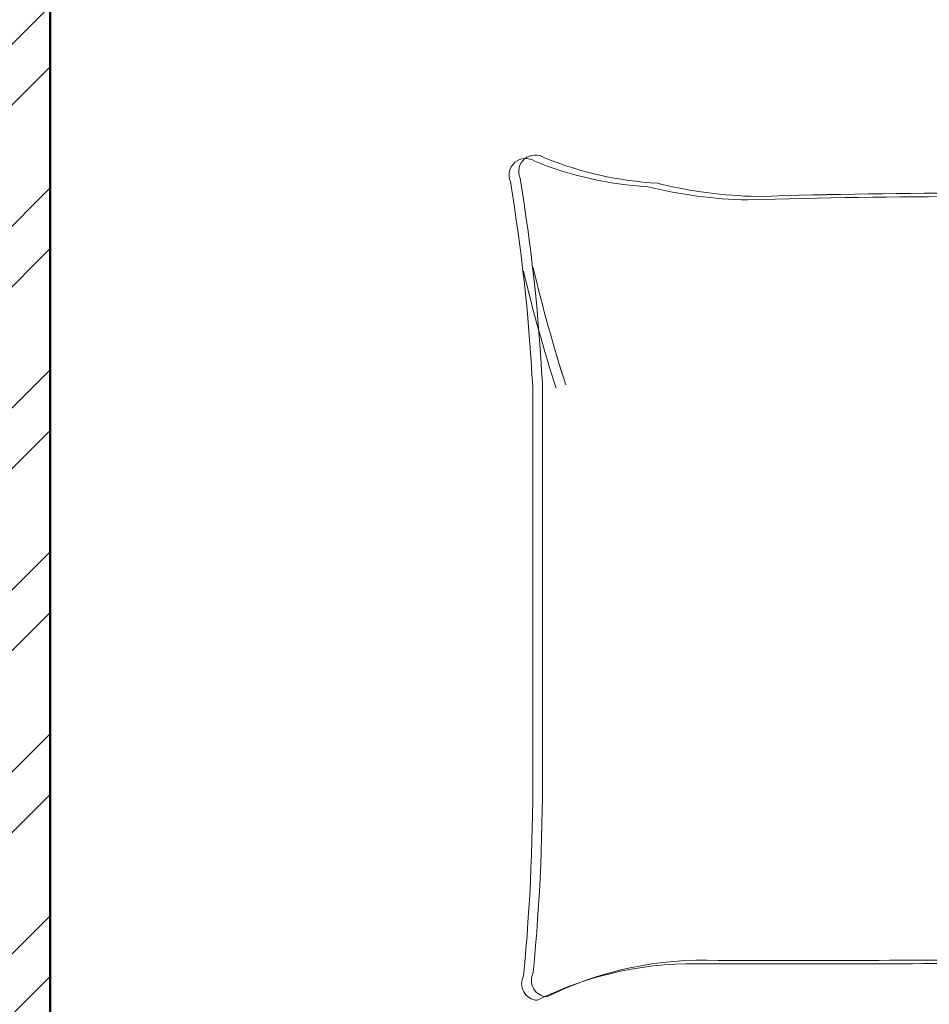
# Model space of a CAD drawing. Units: inches. Extents: x 1901 to 2863, y 888 to 2433.
# Tile 41 of 91: x 2618 to 2686, y 1563 to 1636. Entities that reach past the tile are written whole.
import ezdxf

# ---------------------------------------------------------------- set-up
doc = ezdxf.new("R2010")
doc.units = ezdxf.units.IN
for name, color, linetype, lineweight in [('A-FURN', 8, 'Continuous', 18), ('A-WALL', 7, 'Continuous', 50), ('A-WALL-PATT', 8, 'Continuous', 13)]:
    doc.layers.add(name, color=color, linetype=linetype, lineweight=lineweight)

# ---------------------------------------------------------------- blocks, each defined once
blk = doc.blocks.new('BED-DOUBLE')
for p, q in [((31.178, 59.321), (27.529, 55.161)), ((31.178, 59.32), (27.529, 55.16)), ((31.896, 59.577), (28.246, 55.417)), ((31.896, 59.577), (28.246, 55.417)), ((33.137, 59.41), (31.178, 59.321, 4.346)), ((33.137, 59.41), (31.178, 59.32, 4.346)), ((31.873, 57.595), (31.178, 59.321)), ((31.873, 57.595), (31.178, 59.32)), ((33.854, 59.666), (31.896, 59.577, 4.346)), ((33.854, 59.666), (31.896, 59.577, 4.346)), ((32.591, 57.851), (31.896, 59.577)), ((32.591, 57.851), (31.896, 59.577)), ((0.026, 57.778), (0.026, 4.122)), ((0.744, 57.778), (30.62, 57.778)), ((0.744, 57.778), (30.62, 57.778)), ((31.525, 54.117), (31.873, 57.595)), ((31.525, 54.117), (31.873, 57.595)), ((32.243, 54.374), (32.591, 57.851)), ((32.243, 54.373), (32.591, 57.851)), ((18.633, 56.885), (15.109, 56.014)), ((18.633, 56.885), (15.109, 56.014)), ((19.351, 57.142), (15.827, 56.271)), ((19.351, 57.141), (15.827, 56.271)), ((18.18, 51.123), (18.633, 56.885)), ((18.18, 51.123), (18.633, 56.885)), ((18.898, 51.38), (19.351, 57.142)), ((18.898, 51.379), (19.351, 57.141)), ((2.897, 56.227), (2.788, 50.161)), ((2.897, 56.227), (2.788, 50.161)), ((2.897, 56.227), (6.502, 55.801)), ((2.897, 56.227), (6.502, 55.802)), ((3.615, 56.483), (3.506, 50.417)), ((3.615, 56.483), (3.506, 50.418)), ((3.615, 56.483), (7.22, 56.058)), ((3.615, 56.483), (7.22, 56.058)), ((6.502, 55.801), (9.388, 56.47)), ((6.502, 55.802), (9.388, 56.47)), ((7.22, 56.058), (10.106, 56.726)), ((7.22, 56.058), (10.106, 56.726)), ((13.307, 56.227), (9.297, 55.326)), ((13.307, 56.227), (9.297, 55.326)), ((9.388, 56.47), (10.563, 55.893)), ((9.388, 56.47), (10.563, 55.893)), ((14.025, 56.483), (10.015, 55.582)), ((14.025, 56.483), (10.015, 55.582)), ((10.106, 56.726), (11.28, 56.149)), ((10.106, 56.726), (11.28, 56.149)), ((15.109, 56.014), (13.307, 56.227)), ((15.109, 56.014), (13.307, 56.227)), ((15.827, 56.271), (14.025, 56.483)), ((15.827, 56.271), (14.025, 56.483)), ((10.015, 55.582), (7.007, 54.256)), ((10.015, 55.582), (7.007, 54.256)), ((28.246, 55.417), (25.814, 52.113)), ((28.246, 55.417), (25.814, 52.113)), ((9.297, 55.326), (6.289, 53.999)), ((9.297, 55.326), (6.289, 54)), ((27.529, 55.161), (25.096, 51.857)), ((27.529, 55.16), (25.096, 51.856)), ((31.873, 49.77), (31.525, 54.117)), ((31.873, 49.77), (31.525, 54.117)), ((32.591, 50.027), (32.243, 54.374)), ((32.591, 50.026), (32.243, 54.373)), ((25.096, 51.857), (22.837, 45.597)), ((25.096, 51.856), (22.837, 45.597)), ((25.814, 52.113), (23.554, 45.853)), ((25.814, 52.113), (23.554, 45.853)), ((2.788, 50.161), (2.881, 51.287)), ((2.788, 50.161), (2.881, 51.287)), ((2.881, 51.287), (3.472, 47.023)), ((2.881, 51.287), (3.472, 47.023)), ((3.506, 50.418), (3.598, 51.544)), ((3.506, 50.417), (3.598, 51.543)), ((3.598, 51.544), (4.19, 47.279)), ((3.598, 51.543), (4.19, 47.279)), ((18.806, 48.922), (18.18, 51.123)), ((18.806, 48.922), (18.18, 51.123)), ((19.523, 49.179), (18.898, 51.38)), ((19.523, 49.179), (18.898, 51.379)), ((32.394, 45.945), (31.873, 49.77)), ((32.394, 45.944), (31.873, 49.77)), ((33.112, 46.201), (32.591, 50.027)), ((33.112, 46.201), (32.591, 50.026)), ((18.322, 41.052), (18.806, 48.922)), ((18.322, 41.052), (18.806, 48.922)), ((19.039, 41.308), (19.523, 49.179)), ((19.039, 41.308), (19.523, 49.179)), ((3.472, 47.023), (4.991, 40.938)), ((3.472, 47.023), (4.991, 40.938)), ((4.19, 47.279), (5.709, 41.195)), ((4.19, 47.279), (5.709, 41.195)), ((33.437, 43.684), (32.394, 45.945)), ((33.437, 43.684), (32.394, 45.944)), ((34.155, 43.941), (33.112, 46.201)), ((34.155, 43.94), (33.112, 46.201)), ((22.837, 45.597), (19.543, 36.235)), ((22.837, 45.597), (19.543, 36.235)), ((23.554, 45.853), (20.261, 36.492)), ((23.554, 45.853), (20.261, 36.491)), ((88.998, 16.876), (88.998, 44.511)), ((88.998, 16.876), (88.998, 44.511)), ((89.716, 17.132), (89.716, 44.768)), ((89.716, 17.132), (89.716, 44.767)), ((4.151, 43.976), (3.482, 41.657)), ((4.151, 43.975), (3.482, 41.657)), ((4.869, 44.232), (4.2, 41.913)), ((4.869, 44.232), (4.2, 41.914)), ((34.85, 41.158), (34.155, 43.941)), ((34.85, 41.158), (34.155, 43.94)), ((34.132, 40.902), (33.437, 43.684)), ((34.132, 40.902), (33.437, 43.684)), ((3.482, 41.657), (2.875, 38.367)), ((3.482, 41.657), (2.875, 38.367)), ((4.2, 41.914), (3.593, 38.623)), ((4.2, 41.913), (3.593, 38.623)), ((17.573, 36.525), (18.322, 41.052)), ((17.573, 36.525), (18.322, 41.052)), ((18.291, 36.782), (19.039, 41.308)), ((18.291, 36.781), (19.039, 41.308)), ((31.873, 40.554), (34.132, 40.902)), ((31.873, 40.554), (34.132, 40.902)), ((32.591, 40.811), (34.85, 41.158)), ((32.591, 40.81), (34.85, 41.158)), ((26.834, 38.642), (31.873, 40.554)), ((26.834, 38.641), (31.873, 40.554)), ((27.551, 38.898), (32.591, 40.811)), ((27.551, 38.898), (32.591, 40.81)), ((19.543, 33.937), (26.834, 38.642)), ((19.543, 33.937), (26.834, 38.641)), ((20.261, 34.194), (27.551, 38.898)), ((20.261, 34.193), (27.551, 38.898)), ((2.875, 38.367), (2.897, 38.006)), ((2.875, 38.367), (2.897, 38.007)), ((2.897, 38.007), (3.371, 33.035)), ((2.897, 38.006), (3.371, 33.035)), ((3.593, 38.623), (3.615, 38.263)), ((3.593, 38.623), (3.615, 38.263)), ((3.615, 38.263), (4.088, 33.291)), ((3.615, 38.263), (4.088, 33.291)), ((18.82, 34.489), (17.378, 37.936)), ((18.82, 34.488), (17.378, 37.936)), ((19.538, 34.745), (18.096, 38.192)), ((19.538, 34.745), (18.096, 38.192)), ((18.993, 31.735), (18.82, 34.489)), ((18.993, 31.734), (18.82, 34.488)), ((19.71, 31.991), (19.538, 34.745)), ((19.71, 31.991), (19.538, 34.745)), ((3.371, 33.035), (2.824, 31.374)), ((3.371, 33.035), (2.824, 31.375)), ((4.088, 33.291), (3.542, 31.631)), ((4.088, 33.291), (3.542, 31.631)), ((2.824, 31.375), (8.859, 31.101)), ((2.824, 31.374), (8.859, 31.101)), ((3.542, 31.631), (9.577, 31.358)), ((3.542, 31.631), (9.577, 31.358)), ((9.577, 31.358), (13.182, 30.933)), ((9.577, 31.358), (13.182, 30.932)), ((13.922, 30.767), (15.988, 31.547)), ((13.922, 30.767), (15.988, 31.547)), ((14.64, 31.024), (16.706, 31.803)), ((14.64, 31.024), (16.706, 31.803)), ((15.988, 31.547), (18.993, 31.735)), ((15.988, 31.547), (18.993, 31.734)), ((16.706, 31.803), (19.71, 31.991)), ((16.706, 31.803), (19.71, 31.991)), ((8.85, 30.041), (12.422, 30.69)), ((8.85, 30.041), (12.422, 30.69)), ((8.859, 31.101), (12.464, 30.676)), ((8.859, 31.101), (12.464, 30.676)), ((12.422, 30.69), (13.883, 30.69)), ((12.422, 30.69), (13.883, 30.69)), ((12.464, 30.676), (13.922, 30.767)), ((12.464, 30.676), (13.922, 30.767)), ((13.182, 30.932), (14.64, 31.024)), ((13.182, 30.933), (14.64, 31.024)), ((13.883, 30.69), (15.993, 30.041)), ((13.883, 30.69), (15.993, 30.041)), ((2.844, 29.392), (8.85, 30.041)), ((2.844, 29.392), (8.85, 30.041)), ((8.132, 29.785), (11.704, 30.434)), ((8.132, 29.784), (11.704, 30.434)), ((11.704, 30.434), (13.165, 30.434)), ((11.704, 30.434), (13.165, 30.434)), ((13.165, 30.434), (15.275, 29.785)), ((13.165, 30.434), (15.275, 29.784)), ((15.993, 30.041), (19.003, 30.041)), ((15.993, 30.041), (19.003, 30.041)), ((19.003, 30.041), (19.003, 27.282)), ((19.003, 30.041), (19.003, 27.282)), ((2.126, 29.136), (8.132, 29.785)), ((2.126, 29.135), (8.132, 29.784)), ((3.493, 27.769), (2.844, 29.392)), ((3.493, 27.769), (2.844, 29.392)), ((15.275, 29.785), (18.286, 29.785)), ((15.275, 29.784), (18.286, 29.784)), ((18.286, 29.785), (18.286, 27.026)), ((18.286, 29.784), (18.286, 27.025)), ((2.775, 27.513), (2.126, 29.136)), ((2.775, 27.512), (2.126, 29.135)), ((3.331, 22.777), (3.493, 27.769)), ((3.331, 22.778), (3.493, 27.769)), ((18.898, 21.983), (19.351, 27.745)), ((18.898, 21.983), (19.351, 27.745)), ((2.613, 22.521), (2.775, 27.513)), ((2.613, 22.521), (2.775, 27.512)), ((18.286, 27.026), (17.061, 23.495)), ((18.286, 27.025), (17.061, 23.495)), ((19.003, 27.282), (17.779, 23.752)), ((19.003, 27.282), (17.779, 23.751)), ((18.18, 21.727), (18.633, 27.489)), ((18.18, 21.727), (18.633, 27.488)), ((3.331, 22.417), (3.331, 22.778)), ((3.331, 22.416), (3.331, 22.777)), ((2.613, 22.16), (2.613, 22.521)), ((2.613, 22.16), (2.613, 22.521)), ((3.425, 18.914), (2.613, 22.16)), ((3.425, 18.914), (2.613, 22.16)), ((4.142, 19.171), (3.331, 22.417)), ((4.142, 19.17), (3.331, 22.416)), ((19.523, 19.782), (18.898, 21.983)), ((19.523, 19.782), (18.898, 21.983)), ((18.806, 19.526), (18.18, 21.727)), ((18.806, 19.526), (18.18, 21.727)), ((3.749, 13.558), (4.886, 19.726)), ((3.749, 13.558), (4.886, 19.725)), ((4.467, 13.815), (5.603, 19.982)), ((4.467, 13.814), (5.603, 19.982)), ((19.039, 11.912), (19.523, 19.782)), ((19.039, 11.912), (19.523, 19.782)), ((4.954, 16.898), (4.142, 19.171)), ((4.954, 16.898), (4.142, 19.17)), ((18.322, 11.656), (18.806, 19.526)), ((18.322, 11.655), (18.806, 19.526)), ((4.236, 16.642), (3.425, 18.914)), ((4.236, 16.642), (3.425, 18.914)), ((3.425, 9.265), (3.749, 13.558)), ((3.425, 9.265), (3.749, 13.558)), ((4.142, 9.522), (4.467, 13.815)), ((4.142, 9.522), (4.467, 13.814)), ((18.291, 7.385), (19.039, 11.912)), ((18.291, 7.385), (19.039, 11.912)), ((19.039, 11.912), (19.402, 10.639)), ((19.039, 11.912), (19.402, 10.64)), ((17.573, 7.129), (18.322, 11.656)), ((17.573, 7.128), (18.322, 11.655)), ((18.322, 11.656), (18.684, 10.383)), ((18.322, 11.655), (18.684, 10.383)), ((18.684, 10.383), (19.496, 4.661)), ((18.684, 10.383), (19.496, 4.661)), ((19.402, 10.64), (20.214, 4.917)), ((19.402, 10.639), (20.214, 4.917)), ((4.122, 9.403), (4.142, 9.522)), ((4.122, 9.404), (4.142, 9.522)), ((3.404, 9.147), (3.425, 9.265)), ((3.404, 9.147), (3.425, 9.265)), ((3.774, 4.341), (3.404, 9.147)), ((3.774, 4.341), (3.404, 9.147)), ((4.492, 4.597), (4.122, 9.404)), ((4.492, 4.597), (4.122, 9.403)), ((10.08, 5.635), (6.996, 6.771)), ((10.08, 5.634), (6.996, 6.771)), ((10.798, 5.891), (7.714, 7.027)), ((10.798, 5.891), (7.714, 7.027)), ((14.857, 5.242), (10.798, 5.891)), ((14.857, 5.242), (10.798, 5.891)), ((4.467, 4.592), (8.039, 5.242)), ((4.467, 4.593), (8.038, 5.242)), ((8.038, 5.242), (10.961, 4.755)), ((8.039, 5.242), (10.961, 4.755)), ((14.139, 4.986), (10.08, 5.635)), ((14.139, 4.985), (10.08, 5.634)), ((10.243, 4.498), (11.379, 5.148)), ((10.243, 4.499), (11.379, 5.148)), ((10.961, 4.755), (12.097, 5.404)), ((10.961, 4.755), (12.097, 5.404)), ((15.925, 5.31), (14.139, 4.985)), ((15.924, 5.31), (14.139, 4.986)), ((16.642, 5.567), (14.857, 5.242)), ((16.642, 5.566), (14.857, 5.242)), ((19.496, 4.661), (15.924, 5.31)), ((19.496, 4.661), (15.925, 5.31)), ((20.214, 4.917), (16.642, 5.567)), ((20.214, 4.917), (16.642, 5.566)), ((3.749, 4.336), (7.321, 4.986)), ((3.749, 4.336), (7.321, 4.985)), ((7.321, 4.986), (10.243, 4.499)), ((7.321, 4.985), (10.243, 4.498))]:
    blk.add_line(p, q)
for centre, radius, start, end in [((77.121, 85.469), 25.896, 267.47137, 296.46809), ((77.121, 85.469), 25.896, 267.47137, 296.46809), ((77.839, 85.726), 25.896, 267.47137, 296.46809), ((77.839, 85.725), 25.896, 267.47137, 296.46809), ((88.578, 61.052), 1.238, 332.65876, 86.02002), ((88.578, 61.052), 1.238, 332.65876, 86.02002), ((89.295, 61.309), 1.238, 332.65876, 86.02002), ((89.295, 61.308), 1.238, 332.65876, 86.02002), ((239.077, 46.423), 149.37, 174.4998, 180.63509), ((239.077, 46.423), 149.37, 174.4998, 180.63509), ((41.517, 204.859), 145.395, 266.97912, 273.83645), ((41.517, 204.859), 145.395, 266.97912, 273.83645), ((76.89, -5061.969), 5121.824, 90.002168, 90.286888), ((76.89, -5061.97), 5121.824, 90.002168, 90.286888), ((238.36, 46.167), 149.37, 174.4998, 180.63509), ((238.36, 46.167), 149.37, 174.4998, 180.63509), ((-7.447, 57.591), 40.624, 349.87628, 2.56571), ((-7.447, 57.591), 40.624, 349.87628, 2.56571), ((40.799, 204.603), 145.395, 266.97912, 273.83645), ((40.799, 204.602), 145.395, 266.97912, 273.83645), ((-6.729, 57.848), 40.624, 349.87628, 2.56571), ((-6.729, 57.847), 40.624, 349.87628, 2.56571), ((76.173, -5062.226), 5121.824, 90.002168, 90.286888), ((76.173, -5062.226), 5121.824, 90.002168, 90.286888), ((39.397, 49.077), 6.988, 168.6608, 203.73842), ((39.397, 49.076), 6.988, 168.6608, 203.73842), ((40.115, 49.333), 6.988, 168.6608, 203.73842), ((40.115, 49.333), 6.988, 168.6608, 203.73842), ((1.69, 34.942), 33.294, 10.66171, 19.88058), ((1.69, 34.941), 33.294, 10.66171, 19.88058), ((2.408, 35.198), 33.294, 10.66171, 19.88058), ((2.408, 35.198), 33.294, 10.66171, 19.88058), ((176.248, 20.155), 144.857, 171.78449, 186.90062), ((176.248, 20.155), 144.857, 171.78449, 186.90062), ((34.202, 41.097), 0.207, 250.24637, 1.13765), ((34.202, 41.097), 0.207, 250.24637, 1.13765), ((34.92, 41.353), 0.207, 250.24637, 1.13765), ((34.92, 41.353), 0.207, 250.24637, 1.13765), ((175.53, 19.899), 144.857, 171.78449, 186.90062), ((175.53, 19.899), 144.857, 171.78449, 186.90062), ((204.426, 23.944), 185.219, 176.08655, 186.78213), ((204.426, 23.944), 185.219, 176.08655, 186.78213), ((205.143, 24.201), 185.219, 176.08655, 186.78213), ((205.143, 24.2), 185.219, 176.08655, 186.78213), ((225.516, 24.021), 136.704, 182.99578, 189.40907), ((225.516, 24.02), 136.704, 182.99578, 189.40907), ((226.234, 24.277), 136.704, 182.99578, 189.40907), ((226.234, 24.277), 136.704, 182.99578, 189.40907), ((35.026, -187.881), 190.991, 88.4762, 91.00819), ((35.026, -187.881), 190.991, 88.4762, 91.00819), ((35.744, -187.624), 190.991, 88.4762, 91.00819), ((35.744, -187.625), 190.991, 88.4762, 91.00819), ((56.853, 544.298), 541.514, 268.22771, 271.71854), ((56.853, 544.297), 541.514, 268.22771, 271.71854), ((57.571, 544.554), 541.514, 268.22771, 271.71854), ((57.571, 544.554), 541.514, 268.22771, 271.71854), ((72.461, -30.238), 33.271, 76.06484, 88.91125), ((72.461, -30.238), 33.271, 76.06484, 88.91125), ((73.178, -29.981), 33.271, 76.06484, 88.91125), ((73.178, -29.982), 33.271, 76.06484, 88.91125), ((22.589, 95.579), 93.531, 268.72178, 275.60397), ((22.589, 95.579), 93.531, 268.72178, 275.60397), ((23.307, 95.835), 93.531, 268.72178, 275.60397), ((23.307, 95.835), 93.531, 268.72178, 275.60397), ((79.646, -24.098), 26.454, 67.97508, 86.652), ((79.646, -24.098), 26.454, 67.97508, 86.652), ((78.928, -24.355), 26.454, 67.97508, 86.652), ((78.928, -24.355), 26.454, 67.97508, 86.652), ((89.529, 1.185), 1.223, 236.17358, 23.47814), ((89.529, 1.184), 1.223, 236.17358, 23.47814), ((90.247, 1.441), 1.223, 236.17358, 23.47814), ((90.247, 1.441), 1.223, 236.17358, 23.47814)]:
    blk.add_arc(centre, radius, start, end)

msp = doc.modelspace()

# ---------------------------------------------------------------- hatches: boundary and pattern name
at = {"layer": 'A-WALL-PATT'}
h = msp.add_hatch(dxfattribs=at)
h.set_pattern_fill('ANSI32', color=256)
h.paths.add_polyline_path([(2443.926, 2139.888), (2439.426, 2139.888), (2439.426, 2069.348), (2441.676, 2069.348), (2443.926, 2069.348), (2443.926, 2078.634), (2521.926, 2078.634), (2521.926, 2075.067), (2524.176, 2075.067), (2526.426, 2075.067), (2526.426, 2078.634), (2571.755, 2078.634), (2571.755, 2080.884), (2571.755, 2083.134), (2443.926, 2083.134)])
h.paths.add_polyline_path([(2526.426, 2054.634), (2524.176, 2054.634), (2521.926, 2054.634), (2521.926, 2030.634), (2443.926, 2030.634), (2443.926, 2045.348), (2439.426, 2045.348), (2439.426, 1983.867), (2443.926, 1983.867), (2443.926, 2026.134), (2521.926, 2026.134), (2526.426, 2026.134)])
h.paths.add_polyline_path([(2443.926, 1923.867), (2439.426, 1923.867), (2439.426, 1872.634), (2443.926, 1872.634)])
h.paths.add_polyline_path([(2636.233, 1766.134), (2609.926, 1766.134), (2609.926, 1779.785), (2605.426, 1779.785), (2605.426, 1766.134), (2486.614, 1766.134), (2486.614, 1770.671), (2482.114, 1770.671), (2482.114, 1766.134), (2482.114, 1761.634), (2636.233, 1761.634), (2636.233, 1763.884)])
h.paths.add_polyline_path([(2519.536, 1663.384), (2519.536, 1665.634), (2494.926, 1665.634), (2481.831, 1665.634), (2481.831, 1663.384), (2481.831, 1661.134), (2490.426, 1661.134), (2490.426, 1640.157), (2494.926, 1640.157), (2494.926, 1661.134), (2519.536, 1661.134)])
h.paths.add_polyline_path([(2443.926, 1712.134), (2443.926, 1716.634), (2414.464, 1716.634), (2414.464, 1712.134), (2439.426, 1712.134), (2439.426, 1545.507), (2443.926, 1545.507), (2443.926, 1661.134), (2448.475, 1661.134), (2448.475, 1665.634), (2443.926, 1665.634)])
h.paths.add_polyline_path([(2343.426, 1712.134), (2365.525, 1712.134), (2365.525, 1714.384), (2365.525, 1716.634), (2333.871, 1716.634), (2333.871, 1714.384), (2333.871, 1712.134), (2338.926, 1712.134), (2338.926, 1575.634), (2338.926, 1545.507), (2343.426, 1545.507), (2343.426, 1547.507), (2343.426, 1580.134)])
h.paths.add_polyline_path([(2752.926, 1665.634), (2579.536, 1665.634), (2579.536, 1661.134), (2615.926, 1661.134), (2615.926, 1529.134), (2598.931, 1529.134), (2598.931, 1524.634), (2623.127, 1524.634), (2623.127, 1526.884), (2623.127, 1529.134), (2620.426, 1529.134), (2620.426, 1661.134), (2748.426, 1661.134), (2748.426, 1633.499), (2752.926, 1633.499)])
h.paths.add_polyline_path([(2752.926, 1419.929), (2748.426, 1419.929), (2748.426, 1400.134), (2659.426, 1400.134), (2659.426, 1444.333), (2657.176, 1444.333), (2654.926, 1444.333), (2654.926, 1400.134), (2643.649, 1400.134), (2643.649, 1395.634), (2748.426, 1395.634), (2748.426, 1364.035), (2752.926, 1364.035)])
h.paths.add_polyline_path([(2752.926, 1492.878), (2748.426, 1492.878), (2748.426, 1476.634), (2667.426, 1476.634), (2667.426, 1479.71), (2665.176, 1479.71), (2662.926, 1479.71), (2662.926, 1476.634), (2654.926, 1476.634), (2654.926, 1469.536), (2659.426, 1469.536), (2659.426, 1472.134), (2748.426, 1472.134), (2748.426, 1455.929), (2752.926, 1455.929)])
h.paths.add_polyline_path([(2752.926, 1304.035), (2748.426, 1304.035), (2748.426, 1263.634), (2738.66, 1263.634), (2738.66, 1259.134), (2752.926, 1259.134)])
h.paths.add_polyline_path([(2685.926, 1259.134), (2695.49, 1259.134), (2695.49, 1261.384), (2695.49, 1263.634), (2677.837, 1263.634), (2677.837, 1261.384), (2677.837, 1259.134), (2681.426, 1259.134), (2681.426, 1203.634), (2653.277, 1203.634), (2653.277, 1199.134), (2685.926, 1199.134), (2685.926, 1203.634)])
h.paths.add_polyline_path([(2609.426, 1395.634), (2611.848, 1395.634), (2611.848, 1400.134), (2598.888, 1400.134), (2598.888, 1397.884), (2598.888, 1395.634), (2604.926, 1395.634), (2604.926, 1268.134), (2554.726, 1268.134), (2554.726, 1265.884), (2554.726, 1263.634), (2604.926, 1263.634), (2604.926, 1203.634), (2571.306, 1203.634), (2571.306, 1199.134), (2604.926, 1199.134), (2629.277, 1199.134), (2629.277, 1201.384), (2629.277, 1203.634), (2609.426, 1203.634), (2609.426, 1258.634), (2609.426, 1259.134), (2654.804, 1259.134), (2654.804, 1263.634), (2609.426, 1263.634)])
h.paths.add_polyline_path([(2443.926, 1304.035), (2439.426, 1304.035), (2439.426, 1259.134), (2443.926, 1259.134), (2456.16, 1259.134), (2456.16, 1261.384), (2456.16, 1263.634), (2443.926, 1263.634)])
h.paths.add_polyline_path([(2525.426, 1263.634), (2531.778, 1263.634), (2531.778, 1268.134), (2520.926, 1268.134), (2520.926, 1263.634), (2511.409, 1263.634), (2511.409, 1259.134), (2520.926, 1259.134), (2520.926, 1199.134), (2547.306, 1199.134), (2547.306, 1201.384), (2547.306, 1203.634), (2525.426, 1203.634)])
h.paths.add_polyline_path([(2443.926, 1434.842), (2439.426, 1434.842), (2439.426, 1364.035), (2441.676, 1364.035), (2443.926, 1364.035)])
h.paths.add_polyline_path([(2567.134, 1400.134), (2443.926, 1400.134), (2443.926, 1395.634), (2567.134, 1395.634)])
h.paths.add_polyline_path([(2443.926, 1545.507), (2439.426, 1545.507), (2439.426, 1494.842), (2443.926, 1494.842)])
h.paths.add_polyline_path([(2494.926, 1553.349), (2492.676, 1553.349), (2490.426, 1553.349), (2490.426, 1524.634), (2494.926, 1524.634), (2525.936, 1524.634), (2525.936, 1526.884), (2525.936, 1529.134), (2494.926, 1529.134)])
h.paths.add_polyline_path([(2752.926, 1573.499), (2748.426, 1573.499), (2748.426, 1529.134), (2657.759, 1529.134), (2657.759, 1524.634), (2662.926, 1524.634), (2662.926, 1498.631), (2667.426, 1498.631), (2667.426, 1524.634), (2748.426, 1524.634), (2748.426, 1516.878), (2752.926, 1516.878)])
h.paths.add_polyline_path([(2038.602, 2237.418), (2080.174, 2237.418), (2080.174, 2256.075), (2038.602, 2256.075)], flags=9)
h.paths.add_polyline_path([(2292.009, 1062.394), (2539.932, 1062.394), (2539.932, 1099.487), (2292.009, 1099.487)], flags=9)
h.paths.add_polyline_path([(2424.91, 1832.253), (2448.513, 1832.253), (2448.513, 1846.678), (2424.91, 1846.678)], flags=9)
h.paths.add_polyline_path([(2359.076, 1832.253), (2382.678, 1832.253), (2382.678, 1846.678), (2359.076, 1846.678)], flags=9)
h.paths.add_polyline_path([(2352.899, 1684.802), (2367.543, 1684.802), (2367.543, 1697.167), (2352.899, 1697.167)], flags=9)
h.paths.add_polyline_path([(2079.288, 1755.826), (2169.024, 1755.826), (2169.024, 1774.372), (2079.288, 1774.372)], flags=9)
h.paths.add_polyline_path([(2404.09, 1373.857), (2404.09, 1463.593), (2385.544, 1463.593), (2385.544, 1373.857)], flags=9)
h.paths.add_polyline_path([(2268.091, 2236.371), (2309.636, 2236.371), (2309.636, 2255.028), (2268.091, 2255.028)], flags=9)
h.paths.add_polyline_path([(2575.96, 1700.951), (2665.696, 1700.951), (2665.696, 1719.498), (2575.96, 1719.498)], flags=9)
h.paths.add_polyline_path([(2302.962, 1878.474), (2329.524, 1878.474), (2329.524, 1888.777), (2302.962, 1888.777)], flags=9)
h.paths.add_polyline_path([(2097.415, 2240.576), (2126.573, 2240.576), (2126.573, 2259.233), (2097.415, 2259.233)], flags=9)
h.paths.add_polyline_path([(2208.725, 2246.124), (2237.882, 2246.124), (2237.882, 2264.781), (2208.725, 2264.781)], flags=9)
h.paths.add_polyline_path([(2038.147, 1925.958), (2076.987, 1925.958), (2076.987, 1944.615), (2038.147, 1944.615)], flags=9)
h.paths.add_polyline_path([(2239.144, 1926.672), (2288.465, 1926.672), (2288.465, 1945.329), (2239.144, 1945.329)], flags=9)
h.paths.add_polyline_path([(2175.429, 2007.33), (2212.356, 2007.33), (2212.356, 2025.987), (2175.429, 2025.987)], flags=9)
h.paths.add_polyline_path([(2225.034, 2091.794), (2263.875, 2091.794), (2263.875, 2110.451), (2225.034, 2110.451)], flags=9)
h.paths.add_polyline_path([(2035.398, 2098.478), (2074.238, 2098.478), (2074.238, 2117.135), (2035.398, 2117.135)], flags=9)
h.paths.add_polyline_path([(2050.102, 2029.209), (2083.26, 2029.209), (2083.26, 2047.866), (2050.102, 2047.866)], flags=9)
h.paths.add_polyline_path([(2069.677, 1956.719), (2098.835, 1956.719), (2098.835, 1975.376), (2069.677, 1975.376)], flags=9)
h.paths.add_polyline_path([(2328.62, 1753.336), (2361.663, 1753.336), (2361.663, 1771.993), (2328.62, 1771.993)], flags=9)
h.paths.add_polyline_path([(2395.162, 2060.888), (2395.162, 2140.654), (2378.676, 2140.654), (2378.676, 2060.888)], flags=9)
h.paths.add_polyline_path([(2463.728, 2059.02), (2492.886, 2059.02), (2492.886, 2077.677), (2463.728, 2077.677)], flags=9)
h.paths.add_polyline_path([(2458.027, 2181.536), (2496.868, 2181.536), (2496.868, 2200.194), (2458.027, 2200.194)], flags=9)
h.paths.add_polyline_path([(2456.855, 2228.831), (2498.401, 2228.831), (2498.401, 2247.488), (2456.855, 2247.488)], flags=9)
h.paths.add_polyline_path([(2527.577, 2243.074), (2556.735, 2243.074), (2556.735, 2261.731), (2527.577, 2261.731)], flags=9)
h.paths.add_polyline_path([(2694.461, 2232.767), (2736.033, 2232.767), (2736.033, 2251.425), (2694.461, 2251.425)], flags=9)
h.paths.add_polyline_path([(2637.821, 2249.225), (2666.979, 2249.225), (2666.979, 2267.882), (2637.821, 2267.882)], flags=9)
h.paths.add_polyline_path([(2623.687, 2183.541), (2662.528, 2183.541), (2662.528, 2202.199), (2623.687, 2202.199)], flags=9)
h.paths.add_polyline_path([(2691.965, 2021.5), (2725.124, 2021.5), (2725.124, 2040.157), (2691.965, 2040.157)], flags=9)
h.paths.add_polyline_path([(2621.043, 1975.912), (2662.335, 1975.912), (2662.335, 1994.569), (2621.043, 1994.569)], flags=9)
h.paths.add_polyline_path([(2479.032, 1927.62), (2519.844, 1927.62), (2519.844, 1946.277), (2479.032, 1946.277)], flags=9)
h.paths.add_polyline_path([(2670.941, 1849.076), (2716.005, 1849.076), (2716.005, 1867.734), (2670.941, 1867.734)], flags=9)
h.paths.add_polyline_path([(2523.613, 1782.956), (2550.175, 1782.956), (2550.175, 1793.26), (2523.613, 1793.26)], flags=9)
h.paths.add_polyline_path([(2450.841, 1207.331), (2492.386, 1207.331), (2492.386, 1225.989), (2450.841, 1225.989)], flags=9)
h.paths.add_polyline_path([(2527.751, 1203.841), (2556.908, 1203.841), (2556.908, 1222.499), (2527.751, 1222.499)], flags=9)
h.paths.add_polyline_path([(2639.111, 1207.2), (2668.268, 1207.2), (2668.268, 1225.857), (2639.111, 1225.857)], flags=9)
h.paths.add_polyline_path([(2692.594, 1218.965), (2734.167, 1218.965), (2734.167, 1237.623), (2692.594, 1237.623)], flags=9)
h.paths.add_polyline_path([(2669.266, 1366.329), (2708.106, 1366.329), (2708.106, 1384.987), (2669.266, 1384.987)], flags=25)
h.paths.add_polyline_path([(2463.313, 1358.031), (2502.153, 1358.031), (2502.153, 1376.688), (2463.313, 1376.688)], flags=9)
h.paths.add_polyline_path([(2494.725, 1449.963), (2531.652, 1449.963), (2531.652, 1468.62), (2494.725, 1468.62)], flags=9)
h.paths.add_polyline_path([(2675.565, 1422.157), (2708.724, 1422.157), (2708.724, 1440.815), (2675.565, 1440.815)], flags=25)
h.paths.add_polyline_path([(2685.634, 1493.891), (2714.792, 1493.891), (2714.792, 1512.548), (2685.634, 1512.548)], flags=9)
h.paths.add_polyline_path([(2686.805, 1529.913), (2725.645, 1529.913), (2725.645, 1548.57), (2686.805, 1548.57)], flags=25)
h.paths.add_polyline_path([(2503.651, 1537.991), (2552.972, 1537.991), (2552.972, 1556.648), (2503.651, 1556.648)], flags=9)
h.paths.add_polyline_path([(2291.713, 1643.504), (2318.275, 1643.504), (2318.275, 1653.807), (2291.713, 1653.807)], flags=9)
h.paths.add_polyline_path([(2450.626, 1610.52), (2477.189, 1610.52), (2477.189, 1620.824), (2450.626, 1620.824)], flags=9)
h.paths.add_polyline_path([(2359.985, 1551.814), (2422.253, 1551.814), (2422.253, 1562.117), (2359.985, 1562.117)], flags=9)
h.paths.add_polyline_path([(2280.106, 1249.006), (2321.651, 1249.006), (2321.651, 1267.663), (2280.106, 1267.663)], flags=9)
h.paths.add_polyline_path([(2164.057, 1274.232), (2193.215, 1274.232), (2193.215, 1292.889), (2164.057, 1292.889)], flags=9)
h.paths.add_polyline_path([(2118.21, 1277.694), (2151.252, 1277.694), (2151.252, 1296.351), (2118.21, 1296.351)], flags=9)
h.paths.add_polyline_path([(2031.946, 1268.529), (2073.519, 1268.529), (2073.519, 1287.187), (2031.946, 1287.187)], flags=9)
h.paths.add_polyline_path([(2050.199, 1409.079), (2089.04, 1409.079), (2089.04, 1427.736), (2050.199, 1427.736)], flags=9)
h.paths.add_polyline_path([(2243.743, 1421.032), (2282.584, 1421.032), (2282.584, 1439.689), (2243.743, 1439.689)], flags=9)
h.paths.add_polyline_path([(2190.746, 1509.769), (2231.558, 1509.769), (2231.558, 1528.426), (2190.746, 1528.426)], flags=9)
h.paths.add_polyline_path([(2058.392, 1475.415), (2091.55, 1475.415), (2091.55, 1494.073), (2058.392, 1494.073)], flags=9)
h.paths.add_polyline_path([(2062.447, 1553.09), (2091.605, 1553.09), (2091.605, 1571.747), (2062.447, 1571.747)], flags=9)
h.paths.add_polyline_path([(2219.524, 1590.365), (2266.147, 1590.365), (2266.147, 1609.022), (2219.524, 1609.022)], flags=9)
h.paths.add_polyline_path([(2041.072, 1584.188), (2079.912, 1584.188), (2079.912, 1602.845), (2041.072, 1602.845)], flags=9)

# ---------------------------------------------------------------- linework, layer by layer
at = {"layer": 'A-FURN'}
for centre in [(2772.486, 1645.392), (2772.486, 1645.391), (2771.768, 1645.135), (2771.768, 1645.135)]:
    msp.add_arc(centre, 119.527, 193.38322, 197.70533, dxfattribs=at)
at = {"layer": 'A-WALL'}
msp.add_line((2620.426, 1661.134), (2620.426, 1529.134), dxfattribs=at)

# ---------------------------------------------------------------- block references
at = {"layer": 'A-FURN', "rotation": 180}
msp.add_blockref('BED-DOUBLE', (2745.89, 1626.019), dxfattribs=at)

doc.saveas('drawing.dxf')
